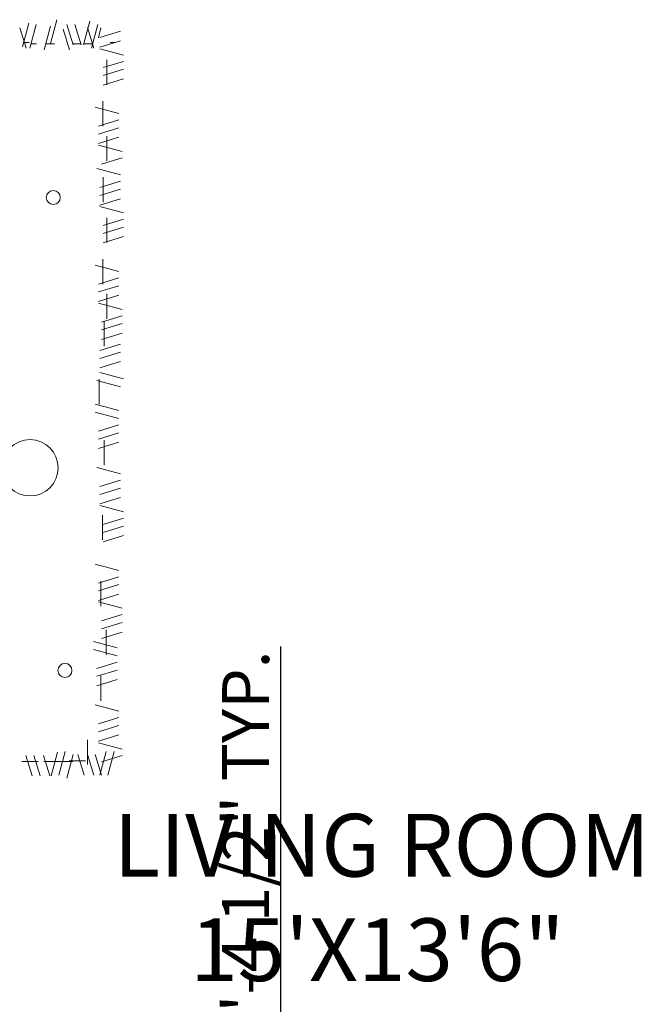
# Model space of a CAD drawing. Units: millimetres. Extents: x 20768 to 23556, y 50760 to 52704.
# Tile 18 of 36: x 21408 to 21487, y 51912 to 52037. Entities that reach past the tile are written whole.
import ezdxf

# ---------------------------------------------------------------- set-up
doc = ezdxf.new("R2010")
doc.units = ezdxf.units.MM
for name, color, linetype, lineweight in [('A-AREA-IDEN', 40, 'Continuous', 18), ('A-FURN', 8, 'Continuous', 18), ('S-ANNO-DIMS', 2, 'Continuous', 18)]:
    doc.layers.add(name, color=color, linetype=linetype, lineweight=lineweight)
doc.styles.get("Standard").update_dxf_attribs({"font": 'arial.ttf'})
doc.dimstyles.new('ISO-25', dxfattribs={"dimtxt": 6, "dimasz": 2.5, "dimexe": 1.25, "dimexo": 0.625, "dimtad": 1, "dimdec": 0, "dimlunit": 3, "dimtxsty": 'Standard', "dimcen": 2.5, "dimadec": 0, "dimazin": 0, "dimtfac": 1, "dimtdec": 0, "dimtmove": 0, "dimatfit": 3, "dimfxl": 1, "dimarcsym": 0})

# ---------------------------------------------------------------- blocks, each defined once
blk = doc.blocks.new('A$C32DD204E')
for p, q in [((2006.3, 3063.8, -685.7), (2029.8, 3152, -685.7)), ((2109.5, 3076.2, -685.7), (2133, 3164.3, -685.7)), ((2233, 3070.3, -685.7), (2256.6, 3158.5, -685.7)), ((2019.3, 3057.9, -685.7), (1995.7, 3134.4, -685.7)), ((2032.9, 3058.5, -685.7), (2056.5, 3146.7, -685.7)), ((2086.3, 3052.6, -685.7), (2109.9, 3140.8, -685.7)), ((2180.5, 3052.6, -685.7), (2156.9, 3129.1, -685.7)), ((2194.3, 3070.3, -685.7), (2170.7, 3146.7, -685.7)), ((2223.7, 3070.3, -685.7), (2200.2, 3146.7, -685.7)), ((2270.6, 3058.5, -685.7), (2247.1, 3134.9, -685.7)), ((2262.4, 3058.5, -685.7), (2286, 3146.7, -685.7)), ((2287.7, 3097.5, -685.7), (2297.5, 3134.4, -685.7)), ((2370, 3121.3, -685.7), (2293.6, 3097.7, -685.7)), ((2370, 3086, -685.7), (2293.6, 3062.4, -685.7)), ((2381.8, 3033, -685.7), (2293.6, 3056.6, -685.7)), ((2381.8, 3009.5, -685.7), (2305.3, 2986, -685.7)), ((2319.2, 3015.1, 685.7), (2319.2, 2922.6, 685.7)), ((2381.8, 2980.1, -685.7), (2305.3, 2956.6, -685.7)), ((2381.8, 2944.8, -685.7), (2305.3, 2921.3, -685.7)), ((2304.1, 2861.1, 685.7), (2304.1, 2768.6, 685.7)), ((2364.1, 2815.4, -685.7), (2275.9, 2838.9, -685.7)), ((2364.1, 2791.8, -685.7), (2287.7, 2768.3, -685.7)), ((2364.1, 2762.4, -685.7), (2287.7, 2738.9, -685.7)), ((2364.1, 2727.1, -685.7), (2287.7, 2703.6, -685.7)), ((2319.2, 2731.6, 685.7), (2319.2, 2639, 685.7)), ((2375.9, 2674.2, -685.7), (2287.7, 2697.7, -685.7)), ((2375.9, 2650.6, -685.7), (2299.4, 2627.1, -685.7)), ((2370, 2586.9, -685.7), (2281.8, 2610.4, -685.7)), ((2305.1, 2578.3), (2305.1, 2485.8)), ((2370, 2563.4, -685.7), (2293.6, 2539.8, -685.7)), ((2370, 2534, -685.7), (2293.6, 2510.4, -685.7)), ((2370, 2498.7, -685.7), (2293.6, 2475.1, -685.7)), ((2381.8, 2445.7, -685.7), (2293.6, 2469.3, -685.7)), ((2381.8, 2422.2, -685.7), (2305.3, 2398.7, -685.7)), ((2319.2, 2427.8, 685.7), (2319.2, 2335.3, 685.7)), ((2381.8, 2392.8, -685.7), (2305.3, 2369.2, -685.7)), ((2381.8, 2357.5, -685.7), (2305.3, 2334, -685.7)), ((2304.1, 2273.8, 685.7), (2304.1, 2181.3, 685.7)), ((2364.1, 2228.1, -685.7), (2275.9, 2251.6, -685.7)), ((2364.1, 2204.5, -685.7), (2287.7, 2181, -685.7)), ((2364.1, 2175.1, -685.7), (2287.7, 2151.6, -685.7)), ((2364.1, 2139.8, -685.7), (2287.7, 2116.3, -685.7)), ((2319.2, 2144.3, 685.7), (2319.2, 2051.7, 685.7)), ((2375.9, 2086.9, -685.7), (2287.7, 2110.4, -685.7)), ((2375.9, 2063.3, -685.7), (2299.4, 2039.8, -685.7)), ((2375.9, 2033.9, -685.7), (2299.4, 2010.4, -685.7)), ((2309.8, 2042.9, 685.7), (2309.8, 1950.3, 685.7)), ((2375.9, 1998.6, -685.7), (2299.4, 1975.1, -685.7)), ((2370, 1957.5, -685.7), (2293.6, 1933.9, -685.7)), ((2370, 1928, -685.7), (2293.6, 1904.5, -685.7)), ((2370, 1892.7, -685.7), (2293.6, 1869.2, -685.7)), ((2381.8, 1828, -685.7), (2293.6, 1851.6, -685.7)), ((2370, 1798.6, -685.7), (2281.8, 1822.1, -685.7)), ((2290.3, 1826.8, 685.7), (2290.3, 1734.2, 685.7)), ((2364.1, 1710.4, -685.7), (2275.9, 1733.9, -685.7)), ((2364.1, 1681, -685.7), (2275.9, 1704.5, -685.7)), ((2364.1, 1657.4, -685.7), (2287.7, 1633.9, -685.7)), ((2364.1, 1628, -685.7), (2287.7, 1604.5, -685.7)), ((2364.1, 1592.7, -685.7), (2287.7, 1569.2, -685.7)), ((2309.8, 1600.2, 685.7), (2309.8, 1507.6, 685.7)), ((2370, 1475.1, -685.7), (2281.8, 1498.6, -685.7)), ((2370, 1451.5, -685.7), (2293.6, 1428, -685.7)), ((2370, 1422.1, -685.7), (2293.6, 1398.6, -685.7)), ((2370, 1386.8, -685.7), (2293.6, 1363.3, -685.7)), ((2381.8, 1333.9, -685.7), (2293.6, 1357.4, -685.7)), ((2303.3, 1321.8, 685.7), (2303.3, 1229.3, 685.7)), ((2381.8, 1310.3, -685.7), (2305.3, 1286.8, -685.7)), ((2381.8, 1280.9, -685.7), (2305.3, 1257.4, -685.7)), ((2381.8, 1245.6, -685.7), (2305.3, 1222.1, -685.7)), ((2364.1, 1116.2, -685.7), (2275.9, 1139.7, -685.7)), ((2364.1, 1092.7, -685.7), (2287.7, 1069.2, -685.7)), ((2364.1, 1063.3, -685.7), (2287.7, 1039.7, -685.7)), ((2296.8, 1075.8, 685.7), (2296.8, 983.2, 685.7)), ((2364.1, 1028, -685.7), (2287.7, 1004.4, -685.7)), ((2375.9, 975, -685.7), (2287.7, 998.6, -685.7)), ((2375.9, 951.5, -685.7), (2299.4, 928, -685.7)), ((2375.9, 922.1, -685.7), (2299.4, 898.6, -685.7)), ((2375.9, 886.8, -685.7), (2299.4, 863.3, -685.7)), ((2316.2, 894.5, 685.7), (2316.2, 802, 685.7)), ((2358.2, 828, -685.7), (2270, 851.5, -685.7)), ((2358.2, 798.5, -685.7), (2270, 822.1, -685.7)), ((2358.2, 775, -685.7), (2281.8, 751.5, -685.7)), ((2358.2, 745.6, -685.7), (2281.8, 722.1, -685.7)), ((2358.2, 710.3, -685.7), (2281.8, 686.8, -685.7)), ((2297.3, 723.5, 685.7), (2297.3, 631, 685.7)), ((2364.1, 592.6, -685.7), (2275.9, 616.2, -685.7)), ((2364.1, 569.1, -685.7), (2287.7, 545.6, -685.7)), ((2364.1, 539.7, -685.7), (2287.7, 516.2, -685.7)), ((2247.2, 486.1, 685.7), (2247.2, 393.6, 685.7)), ((2364.1, 504.4, -685.7), (2287.7, 480.9, -685.7)), ((2136.3, 439.6, -685.7), (2112.8, 351.4, -685.7)), ((2140.9, 354.9, -685.7), (2164.5, 443.1, -685.7)), ((2375.9, 451.5, -685.7), (2287.7, 475, -685.7)), ((2293.8, 354.9, -685.7), (2317.3, 443.1, -685.7)), ((2323.2, 354.9, -685.7), (2346.7, 443.1, -685.7)), ((2003.6, 404.8), (2064.3, 404.8)), ((2018.7, 427.8, -685.7), (2042.2, 351.4, -685.7)), ((2048.1, 427.8, -685.7), (2071.6, 351.4, -685.7)), ((2083.4, 427.8, -685.7), (2106.9, 351.4, -685.7)), ((2084.5, 404.8), (2145.2, 404.8)), ((2131.7, 404.8), (2192.4, 404.8)), ((2170.4, 343.2, -685.7), (2193.9, 431.3, -685.7)), ((2178.9, 408.1), (2239.6, 408.1)), ((2235.1, 354.9, -685.7), (2211.5, 431.3, -685.7)), ((2270.4, 354.9, -685.7), (2246.8, 431.3, -685.7)), ((2299.8, 354.9, -685.7), (2276.2, 431.3, -685.7)), ((2375.9, 427.9, -685.7), (2299.4, 404.4, -685.7))]:
    blk.add_line(p, q)
at = {"elevation": -685.7}
for points in [[(2031.1, 3079.7), (2012.5, 3079.7)], [(2350.5, 3079.7), (2332, 3079.7)], [(2057.7, 3074.4), (2039.2, 3074.4)], [(2124.7, 3074.4), (2092.2, 3074.4)], [(2222.4, 3074.4), (2193, 3074.4)], [(2266.7, 3074.4), (2234.1, 3074.4)], [(2265.7, 3074.4), (2235.6, 3074.4)]]:
    blk.add_lwpolyline(points, dxfattribs=at)
for centre, radius in [((2120.3, 2502.9, -685.7), 26), ((2033.7, 1497.8, -685.7), 104.7), ((2163.6, 744, -685.7), 26)]:
    blk.add_circle(centre, radius)
blk = doc.blocks.new('*D180')
at = {"layer": 'Defpoints', "color": 0, "transparency": 16777216}
for p in [(21434.24, 51900.4), (21441.44, 51900.4), (21434.24, 51895.9)]:
    blk.add_point(p, dxfattribs=at)
at = {"layer": 'S-ANNO-DIMS', "color": 0, "lineweight": -2, "transparency": 16777216}
for p, q in [((21441.44, 51902.9), (21441.44, 51957.2)), ((21434.87, 51900.4), (21442.69, 51900.4)), ((21441.44, 51895.9), (21441.44, 51900.4)), ((21434.87, 51895.9), (21442.69, 51895.9)), ((21441.44, 51893.4), (21441.44, 51890.9))]:
    blk.add_line(p, q, dxfattribs=at)
at = {"layer": 'S-ANNO-DIMS', "color": 0, "transparency": 16777216}
for points in [[(21441.02, 51902.9), (21441.86, 51902.9), (21441.44, 51900.4)], [(21441.02, 51893.4), (21441.86, 51893.4), (21441.44, 51895.9)]]:
    blk.add_solid(points, dxfattribs=at)
at = {"layer": 'S-ANNO-DIMS', "color": 0, "transparency": 16777216, "insert": (21437.71, 51931.3), "char_height": 6, "attachment_point": 5, "rotation": 90}
blk.add_mtext('0\'-4 1/2" TYP.', dxfattribs=at)

msp = doc.modelspace()

# ---------------------------------------------------------------- block references
at = {"layer": 'A-FURN', "xscale": 0.0343301531987817, "yscale": 0.0343301531987817, "zscale": 0.0343301531987817}
msp.add_blockref('A$C32DD204E', (21339.6, 51928.59, 23.54), dxfattribs=at)

# ---------------------------------------------------------------- texts
at = {"layer": 'A-AREA-IDEN', "insert": (21420.09, 51935.81), "char_height": 8, "attachment_point": 1}
msp.add_mtext_dynamic_manual_height_columns('LIVING ROOM\\P    15\'X13\'6"', width=94.7826, gutter_width=12.5, heights=[0], dxfattribs=at)

# ---------------------------------------------------------------- dimensions: what is measured, and where the dimension line sits
at = {"layer": 'S-ANNO-DIMS'}
dim = msp.add_linear_dim(base=(21441.44, 51900.4), p1=(21434.24, 51895.9), p2=(21434.24, 51900.4), angle=90, text='<> TYP.', dimstyle='ISO-25', override={"dimdec": 1, "dimrnd": 0, "dimzin": 1, "dimlunit": 4, "dimfrac": 2}, dxfattribs=at)
dim.commit()
dim.dimension.update_dxf_attribs({"geometry": '*D180', "text_midpoint": (21437.71, 51931.3)})

doc.saveas('drawing.dxf')
